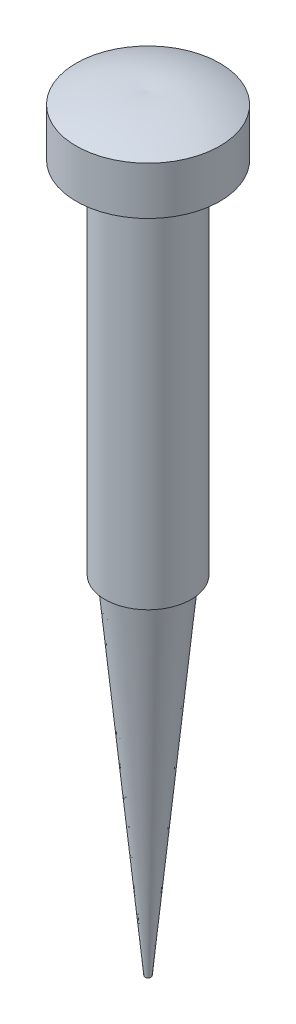
ISO-10303-21;
HEADER;
FILE_DESCRIPTION(('STEP AP214'),'2;1');
FILE_NAME('part.step','',(''),(''),'','','');
FILE_SCHEMA(('AUTOMOTIVE_DESIGN { 1 0 10303 214 1 1 1 1 }'));
ENDSEC;
DATA;
#1=APPLICATION_CONTEXT('core data for automotive mechanical design processes');
#2=APPLICATION_PROTOCOL_DEFINITION('international standard','automotive_design',2000,#1);
#3=PRODUCT_CONTEXT('',#1,'mechanical');
#4=PRODUCT('Part','Part','',(#3));
#5=PRODUCT_RELATED_PRODUCT_CATEGORY('part','',(#4));
#6=PRODUCT_DEFINITION_FORMATION('','',#4);
#7=PRODUCT_DEFINITION_CONTEXT('part definition',#1,'design');
#8=PRODUCT_DEFINITION('design','',#6,#7);
#9=PRODUCT_DEFINITION_SHAPE('','',#8);
#10=(LENGTH_UNIT() NAMED_UNIT(*) SI_UNIT(.MILLI.,.METRE.));
#11=(NAMED_UNIT(*) PLANE_ANGLE_UNIT() SI_UNIT($,.RADIAN.));
#12=(NAMED_UNIT(*) SI_UNIT($,.STERADIAN.) SOLID_ANGLE_UNIT());
#13=UNCERTAINTY_MEASURE_WITH_UNIT(LENGTH_MEASURE(1.E-05),#10,'distance_accuracy_value','');
#14=(GEOMETRIC_REPRESENTATION_CONTEXT(3) GLOBAL_UNCERTAINTY_ASSIGNED_CONTEXT((#13)) GLOBAL_UNIT_ASSIGNED_CONTEXT((#10,
#11,#12)) REPRESENTATION_CONTEXT('',''));
#15=CARTESIAN_POINT('',(0.,0.,0.));
#16=DIRECTION('',(0.,0.,1.));
#17=DIRECTION('',(1.,0.,0.));
#18=AXIS2_PLACEMENT_3D('',#15,#16,#17);
#19=CARTESIAN_POINT('',(1.8,0.,0.));
#20=DIRECTION('',(0.,-1.,0.));
#21=DIRECTION('',(0.,0.,-1.));
#22=AXIS2_PLACEMENT_3D('',#19,#20,#21);
#23=PLANE('',#22);
#24=CARTESIAN_POINT('',(0.,0.,0.));
#25=DIRECTION('',(0.,-1.,0.));
#26=DIRECTION('',(0.,0.,-1.));
#27=AXIS2_PLACEMENT_3D('',#24,#25,#26);
#28=CIRCLE('',#27,1.5);
#29=CARTESIAN_POINT('',(0.,0.,-1.5));
#30=VERTEX_POINT('',#29);
#31=EDGE_CURVE('E11',#30,#30,#28,.T.);
#32=ORIENTED_EDGE('',*,*,#31,.F.);
#33=EDGE_LOOP('',(#32));
#34=FACE_BOUND('',#33,.T.);
#35=CARTESIAN_POINT('',(0.,0.,0.));
#36=DIRECTION('',(0.,-1.,0.));
#37=DIRECTION('',(0.,0.,-1.));
#38=AXIS2_PLACEMENT_3D('',#35,#36,#37);
#39=CIRCLE('',#38,1.8);
#40=CARTESIAN_POINT('',(0.,0.,-1.8));
#41=VERTEX_POINT('',#40);
#42=EDGE_CURVE('E45',#41,#41,#39,.T.);
#43=ORIENTED_EDGE('',*,*,#42,.T.);
#44=EDGE_LOOP('',(#43));
#45=FACE_BOUND('',#44,.T.);
#46=ADVANCED_FACE('F39',(#34,#45),#23,.T.);
#47=CARTESIAN_POINT('',(0.,0.,0.));
#48=DIRECTION('',(0.,-1.,0.));
#49=DIRECTION('',(0.,0.,-1.));
#50=AXIS2_PLACEMENT_3D('',#47,#48,#49);
#51=CYLINDRICAL_SURFACE('',#50,1.8);
#52=CARTESIAN_POINT('',(0.,15.,0.));
#53=DIRECTION('',(0.,-1.,0.));
#54=DIRECTION('',(0.,0.,-1.));
#55=AXIS2_PLACEMENT_3D('',#52,#53,#54);
#56=CIRCLE('',#55,1.8);
#57=CARTESIAN_POINT('',(0.,15.,-1.8));
#58=VERTEX_POINT('',#57);
#59=EDGE_CURVE('E64',#58,#58,#56,.T.);
#60=ORIENTED_EDGE('',*,*,#59,.T.);
#61=EDGE_LOOP('',(#60));
#62=FACE_BOUND('',#61,.T.);
#63=ORIENTED_EDGE('',*,*,#42,.F.);
#64=EDGE_LOOP('',(#63));
#65=FACE_BOUND('',#64,.T.);
#66=ADVANCED_FACE('F74',(#62,#65),#51,.T.);
#67=CARTESIAN_POINT('',(3.,15.,0.));
#68=DIRECTION('',(0.,-1.,0.));
#69=DIRECTION('',(0.,0.,-1.));
#70=AXIS2_PLACEMENT_3D('',#67,#68,#69);
#71=PLANE('',#70);
#72=CARTESIAN_POINT('',(0.,15.,0.));
#73=DIRECTION('',(0.,-1.,0.));
#74=DIRECTION('',(0.,0.,-1.));
#75=AXIS2_PLACEMENT_3D('',#72,#73,#74);
#76=CIRCLE('',#75,3.);
#77=CARTESIAN_POINT('',(0.,15.,-3.));
#78=VERTEX_POINT('',#77);
#79=EDGE_CURVE('E56',#78,#78,#76,.T.);
#80=ORIENTED_EDGE('',*,*,#79,.T.);
#81=EDGE_LOOP('',(#80));
#82=FACE_BOUND('',#81,.T.);
#83=ORIENTED_EDGE('',*,*,#59,.F.);
#84=EDGE_LOOP('',(#83));
#85=FACE_BOUND('',#84,.T.);
#86=ADVANCED_FACE('F77',(#82,#85),#71,.T.);
#87=CARTESIAN_POINT('',(0.,0.,0.));
#88=DIRECTION('',(0.,-1.,0.));
#89=DIRECTION('',(0.,0.,-1.));
#90=AXIS2_PLACEMENT_3D('',#87,#88,#89);
#91=CYLINDRICAL_SURFACE('',#90,3.);
#92=CARTESIAN_POINT('',(0.,17.,0.));
#93=DIRECTION('',(0.,-1.,0.));
#94=DIRECTION('',(0.,0.,-1.));
#95=AXIS2_PLACEMENT_3D('',#92,#93,#94);
#96=CIRCLE('',#95,3.);
#97=CARTESIAN_POINT('',(0.,17.,-3.));
#98=VERTEX_POINT('',#97);
#99=EDGE_CURVE('E60',#98,#98,#96,.T.);
#100=ORIENTED_EDGE('',*,*,#99,.T.);
#101=EDGE_LOOP('',(#100));
#102=FACE_BOUND('',#101,.T.);
#103=ORIENTED_EDGE('',*,*,#79,.F.);
#104=EDGE_LOOP('',(#103));
#105=FACE_BOUND('',#104,.T.);
#106=ADVANCED_FACE('F52',(#102,#105),#91,.T.);
#107=CARTESIAN_POINT('',(0.,11.5248775535342,-0.545812925589026));
#108=DIRECTION('',(-1.,0.,0.));
#109=DIRECTION('',(0.,0.,-1.));
#110=AXIS2_PLACEMENT_3D('',#107,#108,#109);
#111=CIRCLE('',#110,6.);
#112=TRIMMED_CURVE('',#111,(PARAMETER_VALUE(-1.66189108337771)),
(PARAMETER_VALUE(1.66189108337771)),.T.,.PARAMETER.);
#113=CARTESIAN_POINT('',(0.,11.5248775535342,0.));
#114=DIRECTION('',(0.,-1.,0.));
#115=AXIS1_PLACEMENT('',#113,#114);
#116=SURFACE_OF_REVOLUTION('',#112,#115);
#117=CARTESIAN_POINT('',(0.,17.5,0.));
#118=VERTEX_POINT('',#117);
#119=VERTEX_LOOP('',#118);
#120=FACE_BOUND('',#119,.T.);
#121=ORIENTED_EDGE('',*,*,#99,.F.);
#122=EDGE_LOOP('',(#121));
#123=FACE_BOUND('',#122,.T.);
#124=ADVANCED_FACE('F47',(#120,#123),#116,.T.);
#125=CARTESIAN_POINT('',(0.,0.,0.));
#126=DIRECTION('',(0.,1.,0.));
#127=DIRECTION('',(0.,0.,-1.));
#128=AXIS2_PLACEMENT_3D('',#125,#126,#127);
#129=CONICAL_SURFACE('',#128,1.5,0.0945968454580929);
#130=CARTESIAN_POINT('',(0.,-14.5,0.));
#131=DIRECTION('',(0.,-1.,0.));
#132=DIRECTION('',(0.,0.,-1.));
#133=AXIS2_PLACEMENT_3D('',#130,#131,#132);
#134=CIRCLE('',#133,0.124239597669694);
#135=CARTESIAN_POINT('',(0.,-14.5,-0.124239597669695));
#136=VERTEX_POINT('',#135);
#137=EDGE_CURVE('E58',#136,#136,#134,.T.);
#138=CARTESIAN_POINT('',(0.,-14.5,-0.124239597669695));
#139=CARTESIAN_POINT('',(0.,-14.3489583333333,-0.138570435193968));
#140=CARTESIAN_POINT('',(0.,-14.1979166666667,-0.152901272718242));
#141=CARTESIAN_POINT('',(0.,-13.8958333333333,-0.181562947766791));
#142=CARTESIAN_POINT('',(0.,-13.7447916666667,-0.195893785291065));
#143=CARTESIAN_POINT('',(0.,-13.4427083333333,-0.224555460339613));
#144=CARTESIAN_POINT('',(0.,-13.2916666666667,-0.238886297863887));
#145=CARTESIAN_POINT('',(0.,-12.9895833333333,-0.267547972912435));
#146=CARTESIAN_POINT('',(0.,-12.8385416666667,-0.281878810436709));
#147=CARTESIAN_POINT('',(0.,-12.5364583333333,-0.310540485485257));
#148=CARTESIAN_POINT('',(0.,-12.3854166666667,-0.324871323009531));
#149=CARTESIAN_POINT('',(0.,-12.0833333333333,-0.353532998058079));
#150=CARTESIAN_POINT('',(0.,-11.9322916666667,-0.367863835582353));
#151=CARTESIAN_POINT('',(0.,-11.6302083333333,-0.396525510630901));
#152=CARTESIAN_POINT('',(0.,-11.4791666666667,-0.410856348155175));
#153=CARTESIAN_POINT('',(0.,-11.1770833333333,-0.439518023203723));
#154=CARTESIAN_POINT('',(0.,-11.0260416666667,-0.453848860727997));
#155=CARTESIAN_POINT('',(0.,-10.7239583333333,-0.482510535776545));
#156=CARTESIAN_POINT('',(0.,-10.5729166666667,-0.496841373300819));
#157=CARTESIAN_POINT('',(0.,-10.2708333333333,-0.525503048349367));
#158=CARTESIAN_POINT('',(0.,-10.1197916666667,-0.539833885873641));
#159=CARTESIAN_POINT('',(0.,-9.81770833333333,-0.568495560922189));
#160=CARTESIAN_POINT('',(0.,-9.66666666666667,-0.582826398446463));
#161=CARTESIAN_POINT('',(0.,-9.36458333333333,-0.611488073495011));
#162=CARTESIAN_POINT('',(0.,-9.21354166666667,-0.625818911019285));
#163=CARTESIAN_POINT('',(0.,-8.91145833333333,-0.654480586067833));
#164=CARTESIAN_POINT('',(0.,-8.76041666666667,-0.668811423592107));
#165=CARTESIAN_POINT('',(0.,-8.45833333333333,-0.697473098640655));
#166=CARTESIAN_POINT('',(0.,-8.30729166666667,-0.711803936164929));
#167=CARTESIAN_POINT('',(0.,-8.00520833333333,-0.740465611213477));
#168=CARTESIAN_POINT('',(0.,-7.85416666666667,-0.754796448737751));
#169=CARTESIAN_POINT('',(0.,-7.55208333333333,-0.783458123786299));
#170=CARTESIAN_POINT('',(0.,-7.40104166666667,-0.797788961310573));
#171=CARTESIAN_POINT('',(0.,-7.09895833333333,-0.826450636359121));
#172=CARTESIAN_POINT('',(0.,-6.94791666666667,-0.840781473883396));
#173=CARTESIAN_POINT('',(0.,-6.64583333333333,-0.869443148931944));
#174=CARTESIAN_POINT('',(0.,-6.49479166666667,-0.883773986456218));
#175=CARTESIAN_POINT('',(0.,-6.19270833333333,-0.912435661504766));
#176=CARTESIAN_POINT('',(0.,-6.04166666666667,-0.92676649902904));
#177=CARTESIAN_POINT('',(0.,-5.73958333333333,-0.955428174077588));
#178=CARTESIAN_POINT('',(0.,-5.58854166666667,-0.969759011601862));
#179=CARTESIAN_POINT('',(0.,-5.28645833333333,-0.99842068665041));
#180=CARTESIAN_POINT('',(0.,-5.13541666666667,-1.01275152417468));
#181=CARTESIAN_POINT('',(0.,-4.83333333333333,-1.04141319922323));
#182=CARTESIAN_POINT('',(0.,-4.68229166666667,-1.05574403674751));
#183=CARTESIAN_POINT('',(0.,-4.38020833333333,-1.08440571179605));
#184=CARTESIAN_POINT('',(0.,-4.22916666666667,-1.09873654932033));
#185=CARTESIAN_POINT('',(0.,-3.92708333333333,-1.12739822436888));
#186=CARTESIAN_POINT('',(0.,-3.77604166666667,-1.14172906189315));
#187=CARTESIAN_POINT('',(0.,-3.47395833333333,-1.1703907369417));
#188=CARTESIAN_POINT('',(0.,-3.32291666666667,-1.18472157446597));
#189=CARTESIAN_POINT('',(0.,-3.02083333333333,-1.21338324951452));
#190=CARTESIAN_POINT('',(0.,-2.86979166666667,-1.22771408703879));
#191=CARTESIAN_POINT('',(0.,-2.56770833333333,-1.25637576208734));
#192=CARTESIAN_POINT('',(0.,-2.41666666666667,-1.27070659961162));
#193=CARTESIAN_POINT('',(0.,-2.11458333333333,-1.29936827466016));
#194=CARTESIAN_POINT('',(0.,-1.96354166666667,-1.31369911218444));
#195=CARTESIAN_POINT('',(0.,-1.66145833333333,-1.34236078723299));
#196=CARTESIAN_POINT('',(0.,-1.51041666666667,-1.35669162475726));
#197=CARTESIAN_POINT('',(0.,-1.20833333333333,-1.38535329980581));
#198=CARTESIAN_POINT('',(0.,-1.05729166666667,-1.39968413733008));
#199=CARTESIAN_POINT('',(0.,-0.755208333333334,-1.42834581237863));
#200=CARTESIAN_POINT('',(0.,-0.604166666666667,-1.4426766499029));
#201=CARTESIAN_POINT('',(0.,-0.302083333333334,-1.47133832495145));
#202=CARTESIAN_POINT('',(0.,-0.151041666666667,-1.48566916247573));
#203=CARTESIAN_POINT('',(0.,0.,-1.5));
#204=B_SPLINE_CURVE_WITH_KNOTS('',3,(#138,#139,#140,#141,#142,#143,#144,#145,#146,#147,#148,
#149,#150,#151,#152,#153,#154,#155,#156,#157,#158,#159,#160,#161,#162,#163,#164,#165,#166,#167,
#168,#169,#170,#171,#172,#173,#174,#175,#176,#177,#178,#179,#180,#181,#182,#183,#184,#185,#186,
#187,#188,#189,#190,#191,#192,#193,#194,#195,#196,#197,#198,#199,#200,#201,#202,#203),
.UNSPECIFIED.,.F.,.F.,(4,2,2,2,2,2,2,2,2,2,2,2,2,2,2,2,2,2,2,2,2,2,2,2,2,2,2,2,2,2,2,2,4),(0.,
0.455159995784257,0.910319991568514,1.36547998735277,1.82063998313703,2.27579997892128,
2.73095997470554,3.18611997048979,3.64127996627405,4.09643996205831,4.55159995784256,
5.00675995362682,5.46191994941108,5.91707994519533,6.37223994097959,6.82739993676384,
7.2825599325481,7.73771992833236,8.19287992411661,8.64803991990087,9.10319991568512,
9.55835991146938,10.0135199072536,10.4686799030379,10.9238398988222,11.3789998946064,
11.8341598903907,12.2893198861749,12.7444798819592,13.1996398777434,13.6547998735277,
14.1099598693119,14.5651198650962),.UNSPECIFIED.);
#205=EDGE_CURVE('BSEAM55',#136,#30,#204,.T.);
#206=ORIENTED_EDGE('',*,*,#137,.F.);
#207=ORIENTED_EDGE('',*,*,#31,.T.);
#208=ORIENTED_EDGE('',*,*,#205,.T.);
#209=ORIENTED_EDGE('',*,*,#205,.F.);
#210=EDGE_LOOP('',(#206,#208,#207,#209));
#211=FACE_BOUND('',#210,.T.);
#212=ADVANCED_FACE('F55',(#211),#129,.T.);
#213=CARTESIAN_POINT('',(0.,-14.5,0.));
#214=DIRECTION('',(0.,-1.,0.));
#215=DIRECTION('',(0.,0.,-1.));
#216=AXIS2_PLACEMENT_3D('',#213,#214,#215);
#217=PLANE('',#216);
#218=ORIENTED_EDGE('',*,*,#137,.T.);
#219=EDGE_LOOP('',(#218));
#220=FACE_BOUND('',#219,.T.);
#221=ADVANCED_FACE('F90',(#220),#217,.T.);
#222=CLOSED_SHELL('',(#46,#66,#86,#106,#124,#212,#221));
#223=MANIFOLD_SOLID_BREP('B2',#222);
#224=ADVANCED_BREP_SHAPE_REPRESENTATION('',(#18,#223),#14);
#225=SHAPE_DEFINITION_REPRESENTATION(#9,#224);
ENDSEC;
END-ISO-10303-21;
